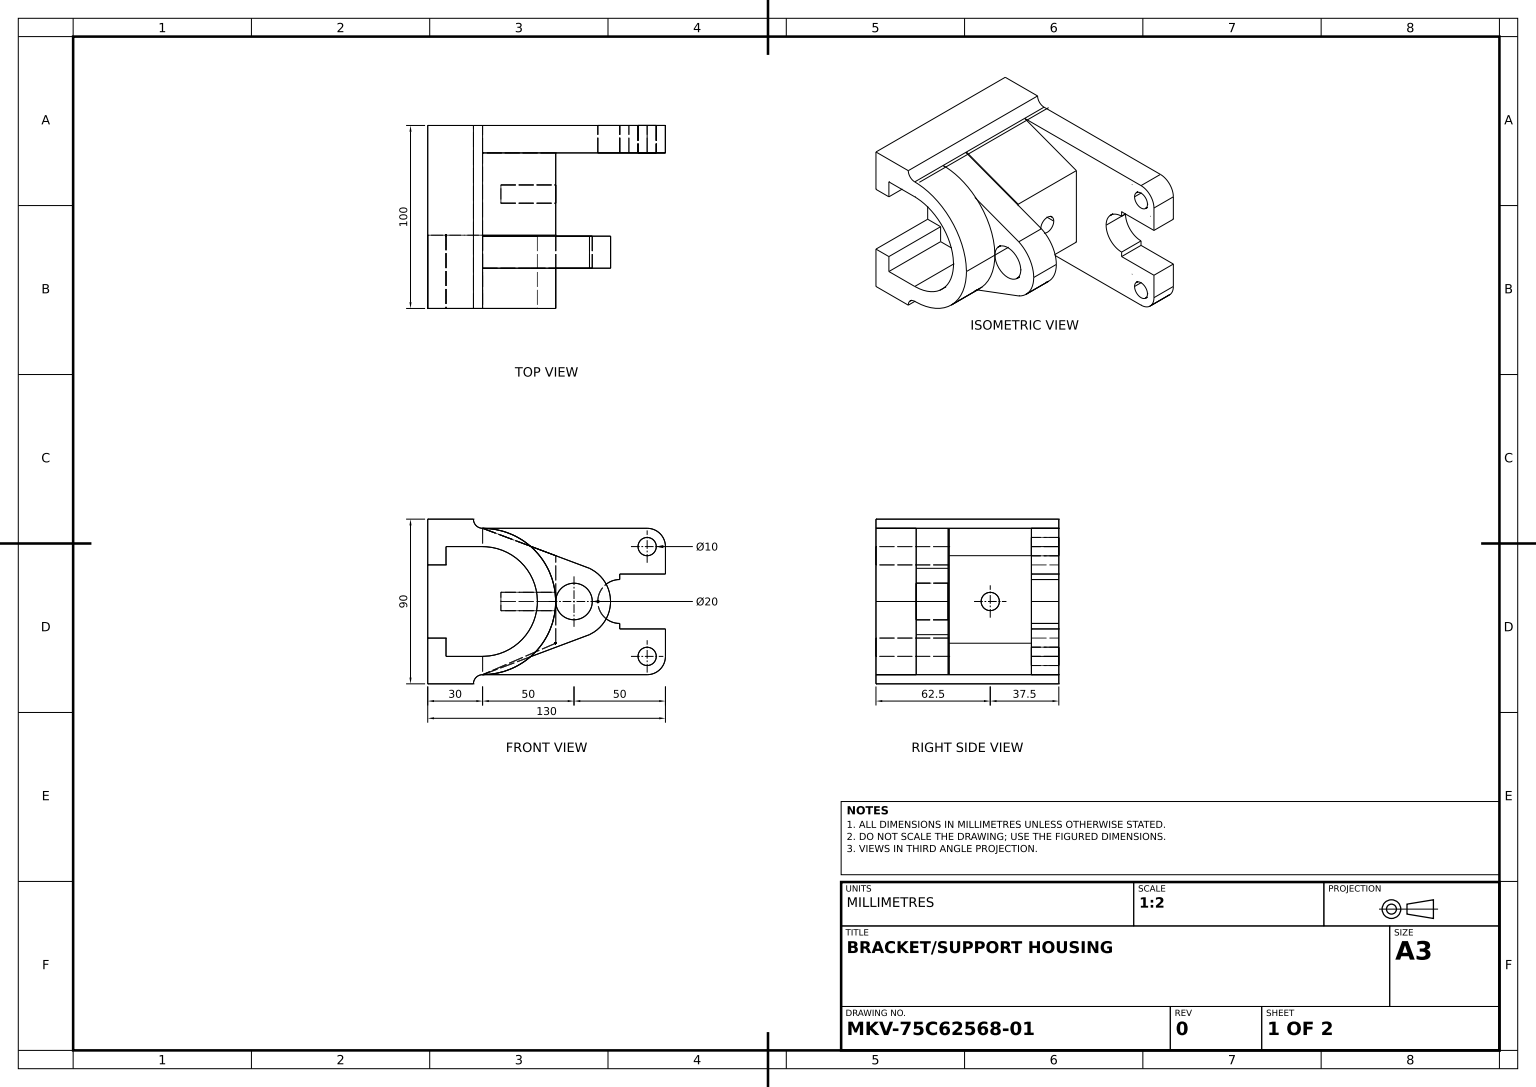
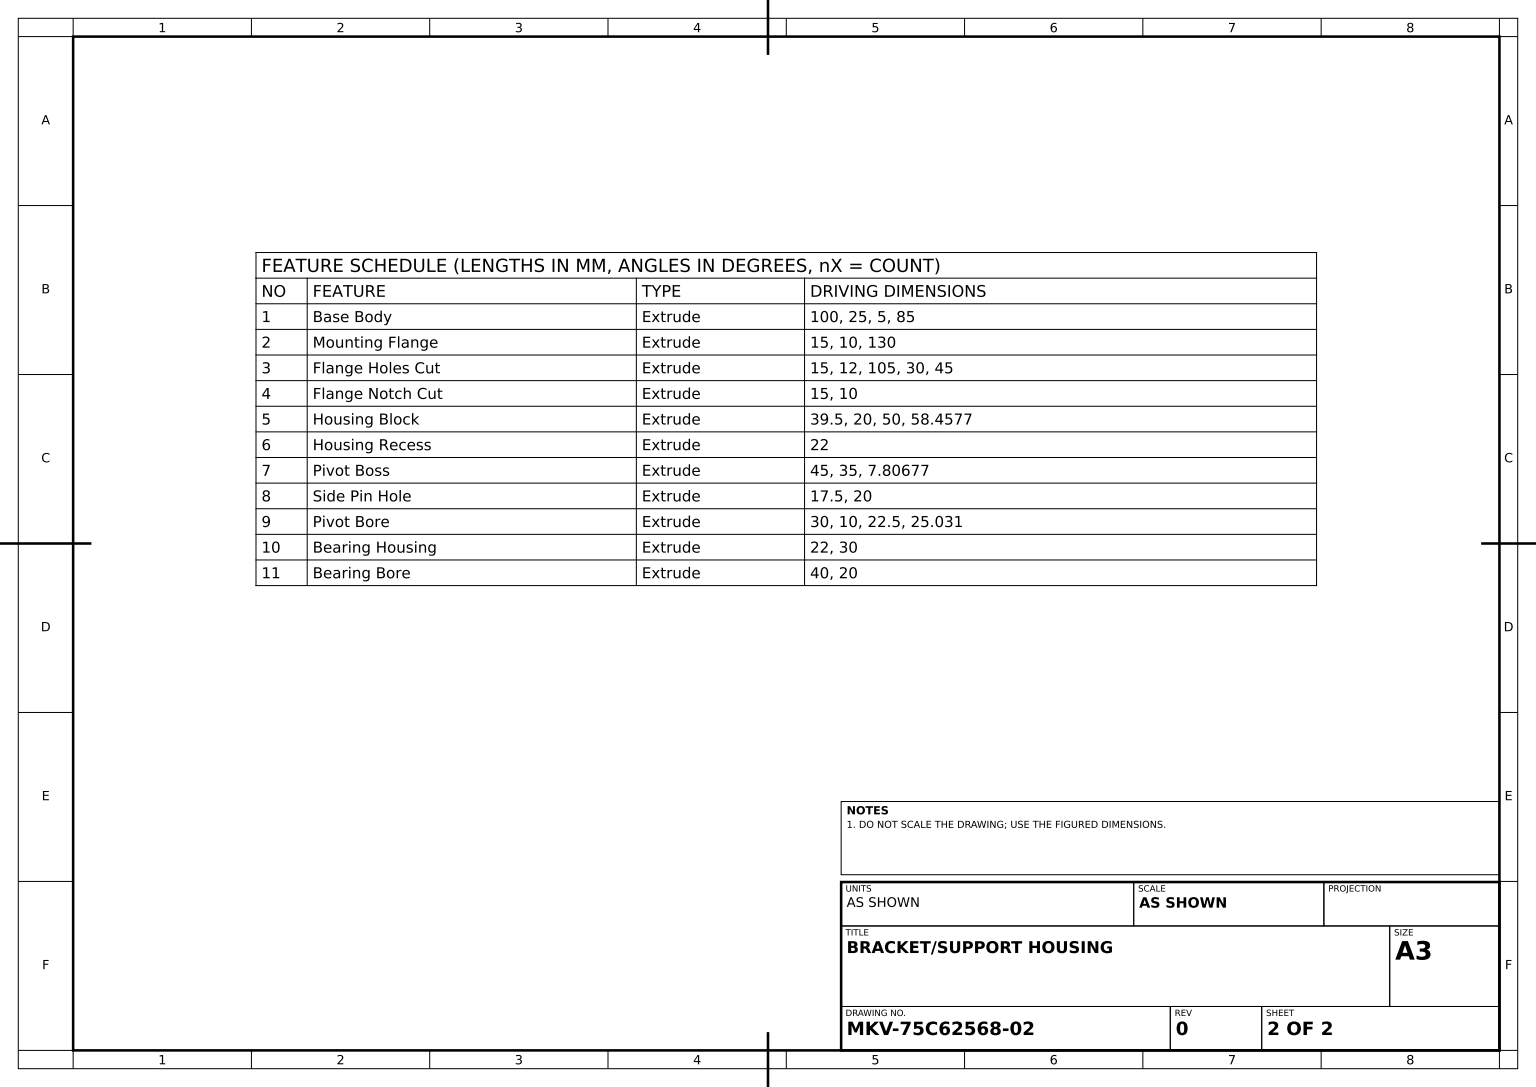
from build123d import *

# Parameters (mm, degrees)
BASE_BODY_DEPTH         = 100
MOUNTING_FLANGE_DEPTH   = 15
FLANGE_HOLES_CUT_DEPTH  = 15
FLANGE_NOTCH_PROFILE_R  = 5
FLANGE_NOTCH_CUT_DEPTH  = 15
HOUSING_BLOCK_DEPTH     = 39.5
HOUSING_RECESS_DEPTH    = 22
PIVOT_BOSS_DEPTH        = 45
SIDE_PIN_HOLE_PROFILE_R = 10
SIDE_PIN_HOLE_DEPTH     = 17.5
PIVOT_BORE_PROFILE_R    = 5
PIVOT_BORE_DEPTH        = 30
BEARING_HOUSING_DEPTH   = 22
BEARING_BORE_DEPTH      = 40


with BuildPart() as part:
    # Base Body Profile → Base Body (new body)
    with BuildSketch(Plane.XY):
        with BuildLine():
            Line((0, 0), (0, 90))
            Line((0, 90), (25, 90))
            ThreePointArc((25, 90), (26.464466094, 86.464466094), (30, 85))
            Line((30, 85), (30, 5))
            ThreePointArc((30, 5), (26.464466094, 3.535533906), (25, 0))
            Line((25, 0), (0, 0))
        make_face()
    extrude(amount=BASE_BODY_DEPTH)

    # Mounting Flange Profile → Mounting Flange (add)
    with BuildSketch(Plane(origin=(0, 0, 0), x_dir=(-1, 0, 0), z_dir=(0, 0, -1))):
        with BuildLine():
            Line((-130, 45), (-130, 75))
            ThreePointArc((-130, 75), (-127.071067812, 82.071067812), (-120, 85))
            Line((-120, 85), (-30, 85))
            Line((-30, 85), (-30, 5))
            Line((-30, 5), (-120, 5))
            ThreePointArc((-120, 5), (-127.071067812, 7.928932188), (-130, 15))
            Line((-130, 15), (-130, 45))
        make_face()
    extrude(amount=-MOUNTING_FLANGE_DEPTH)

    # Flange Holes Profile → Flange Holes Cut (cut)
    with BuildSketch(Plane(origin=(0, 0, 0), x_dir=(-1, 0, 0), z_dir=(0, 0, -1))):
        with BuildLine():
            Line((-130, 60), (-130, 30))
            Line((-130, 30), (-105, 30))
            Line((-105, 30), (-105, 33))
            ThreePointArc((-105, 33), (-93, 45), (-105, 57))
            Line((-105, 57), (-105, 60))
            Line((-105, 60), (-130, 60))
        make_face()
    extrude(amount=-FLANGE_HOLES_CUT_DEPTH, mode=Mode.SUBTRACT)

    # Flange Notch Profile → Flange Notch Cut (cut)
    with BuildSketch(Plane.XY.offset(15)):
        with Locations((120, 75)):
            Circle(FLANGE_NOTCH_PROFILE_R)
        with Locations((120, 15)):
            Circle(FLANGE_NOTCH_PROFILE_R)
    extrude(amount=-FLANGE_NOTCH_CUT_DEPTH, mode=Mode.SUBTRACT)

    # Housing Block Profile → Housing Block (add)
    with BuildSketch(Plane.XY.offset(100)):
        with BuildLine():
            Line((30, 85), (88.457666717, 63.123682675))
            ThreePointArc((88.457666717, 63.123682675), (100, 45), (88.457666717, 26.876317325))
            Line((88.457666717, 26.876317325), (30, 5))
            Line((30, 5), (30, 85))
        make_face()
    extrude(amount=-HOUSING_BLOCK_DEPTH)

    # Housing Recess Profile → Housing Recess (cut)
    with BuildSketch(Plane.XY.offset(100)):
        with BuildLine():
            Line((30, 85), (30, 5))
            Line((30, 5), (88.457666717, 26.876317325))
            ThreePointArc((88.457666717, 26.876317325), (100, 45), (88.457666717, 63.123682675))
            Line((88.457666717, 63.123682675), (30, 85))
        make_face()
    extrude(amount=-HOUSING_RECESS_DEPTH, mode=Mode.SUBTRACT)

    # Pivot Boss Profile → Pivot Boss (add)
    with BuildSketch(Plane.XY.offset(15)):
        Polygon((70, 70.031002054), (30, 85), (30, 45), (70, 45), align=None)
        Polygon((70, 45), (30, 45), (30, 5), (70, 22.19323305), align=None)
    extrude(amount=PIVOT_BOSS_DEPTH)

    # Side Pin Hole Profile → Side Pin Hole (cut)
    with BuildSketch(Plane.XY.offset(78)):
        with Locations((80, 45)):
            Circle(SIDE_PIN_HOLE_PROFILE_R)
    extrude(amount=-SIDE_PIN_HOLE_DEPTH, mode=Mode.SUBTRACT)

    # Pivot Bore Profile → Pivot Bore (cut)
    with BuildSketch(Plane(origin=(70, 0, 0), x_dir=(0, 0, -1), z_dir=(1, 0, 0))):
        with Locations((-37.5, 45)):
            Circle(PIVOT_BORE_PROFILE_R)
    extrude(amount=-PIVOT_BORE_DEPTH, mode=Mode.SUBTRACT)

    # Bearing Housing Profile → Bearing Housing (add)
    with BuildSketch(Plane.XY.offset(100)):
        with BuildLine():
            ThreePointArc((30, 5), (70, 45), (30, 85))
            Line((30, 85), (30, 75))
            ThreePointArc((30, 75), (60, 45), (30, 15))
            Line((30, 15), (30, 5))
        make_face()
    extrude(amount=-BEARING_HOUSING_DEPTH)

    # Bearing Bore Profile → Bearing Bore (cut)
    with BuildSketch(Plane.XY.offset(100)):
        with BuildLine():
            Line((30, 75), (10, 75))
            Line((10, 75), (10, 65))
            Line((10, 65), (0, 65))
            Line((0, 65), (0, 25))
            Line((0, 25), (10, 25))
            Line((10, 25), (10, 15))
            Line((10, 15), (30, 15))
            ThreePointArc((30, 15), (60, 45), (30, 75))
        make_face()
    extrude(amount=-BEARING_BORE_DEPTH, mode=Mode.SUBTRACT)


solid = part.part
